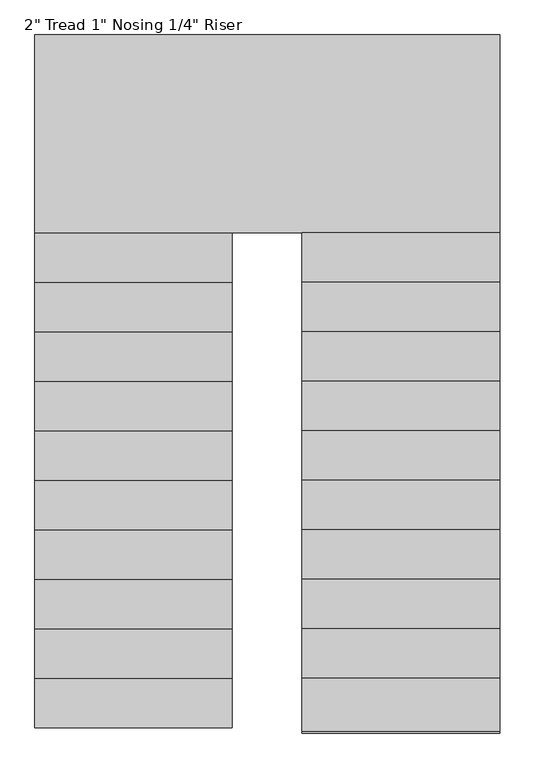
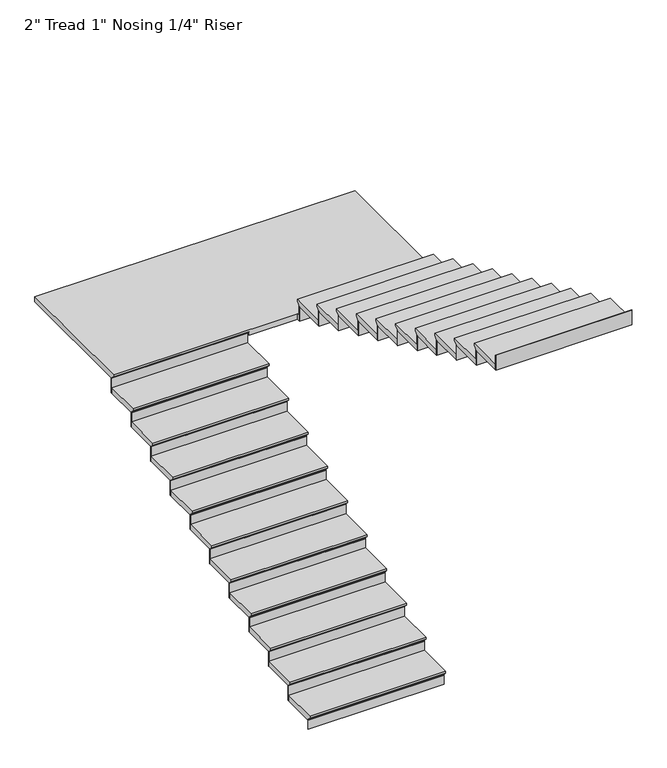
"""IFC4 building model written with IfcOpenShell, lengths in millimetres: stair flight geometry."""

from ifc_helpers import new_model, si_unit, origin, place, context, project, spatial, faceted_brep, source, transform, mapped, element, save


def stair_flight_7b3ce822(model_context):
    return source(origin(), model_context, "Body", "Brep", [
        faceted_brep([(-629.5987998, 3364.6067329, 12921.0954545), (-629.5987998, 3364.6067329, 12940.1454545), (-1845.5417538, 3364.6067329, 12940.1454545), (-1845.5417538, 3364.6067329, 12921.0954545), (-629.5987998, 3390.0067329, 12895.6954545), (-1845.5417538, 3390.0067329, 12895.6954545), (-629.5987998, 3694.8067329, 12940.1454545), (-1845.5417538, 3694.8067329, 12940.1454545), (-1845.5417538, 3390.0067329, 12889.3454545), (-1845.5417538, 3694.8067329, 12889.3454545), (-629.5987998, 3694.8067329, 12889.3454545), (-629.5987998, 3390.0067329, 12889.3454545)], [[[0, 1, 2, 3]], [[4, 0, 3, 5]], [[2, 1, 6, 7]], [[8, 9, 10, 11]], [[2, 7, 9, 8, 5, 3]], [[8, 11, 4, 5]], [[6, 1, 0, 4, 11, 10]], [[7, 6, 10, 9]]]),
        faceted_brep([(-629.5987998, 3390.0067329, 12889.3454545), (-629.5987998, 3390.0067329, 12801.6), (-629.5987998, 3396.3567329, 12801.6), (-629.5987998, 3396.3567329, 12889.3454545), (-1845.5417538, 3390.0067329, 12889.3454545), (-1845.5417538, 3396.3567329, 12889.3454545), (-1845.5417538, 3396.3567329, 12801.6), (-1845.5417538, 3390.0067329, 12801.6)], [[[0, 1, 2, 3]], [[4, 5, 6, 7]], [[1, 0, 4, 7]], [[2, 1, 7, 6]], [[3, 2, 6, 5]], [[0, 3, 5, 4]]]),
        faceted_brep([(-629.5987998, 3694.8067329, 13027.8909091), (-629.5987998, 3694.8067329, 12889.3454545), (-629.5987998, 3701.1567329, 12889.3454545), (-629.5987998, 3701.1567329, 13027.8909091), (-1845.5417538, 3694.8067329, 13027.8909091), (-1845.5417538, 3701.1567329, 13027.8909091), (-1845.5417538, 3701.1567329, 12889.3454545), (-1845.5417538, 3694.8067329, 12889.3454545)], [[[0, 1, 2, 3]], [[4, 5, 6, 7]], [[1, 0, 4, 7]], [[2, 1, 7, 6]], [[3, 2, 6, 5]], [[0, 3, 5, 4]]]),
        faceted_brep([(-1845.5417538, 3669.4067329, 13078.6909091), (-629.5987998, 3669.4067329, 13078.6909091), (-629.5987998, 3999.6067329, 13078.6909091), (-1845.5417538, 3999.6067329, 13078.6909091), (-1845.5417538, 3694.8067329, 13027.8909091), (-1845.5417538, 3999.6067329, 13027.8909091), (-629.5987998, 3999.6067329, 13027.8909091), (-629.5987998, 3694.8067329, 13027.8909091), (-1845.5417538, 3694.8067329, 13034.2409091), (-1845.5417538, 3669.4067329, 13059.6409091), (-629.5987998, 3694.8067329, 13034.2409091), (-629.5987998, 3669.4067329, 13059.6409091)], [[[0, 1, 2, 3]], [[4, 5, 6, 7]], [[0, 3, 5, 4, 8, 9]], [[4, 7, 10, 8]], [[2, 1, 11, 10, 7, 6]], [[3, 2, 6, 5]], [[11, 1, 0, 9]], [[10, 11, 9, 8]]]),
        faceted_brep([(-629.5987998, 3999.6067329, 13166.4363636), (-629.5987998, 3999.6067329, 13027.8909091), (-629.5987998, 4005.9567329, 13027.8909091), (-629.5987998, 4005.9567329, 13166.4363636), (-1845.5417538, 3999.6067329, 13166.4363636), (-1845.5417538, 4005.9567329, 13166.4363636), (-1845.5417538, 4005.9567329, 13027.8909091), (-1845.5417538, 3999.6067329, 13027.8909091)], [[[0, 1, 2, 3]], [[4, 5, 6, 7]], [[1, 0, 4, 7]], [[2, 1, 7, 6]], [[3, 2, 6, 5]], [[0, 3, 5, 4]]]),
        faceted_brep([(-1845.5417538, 3974.2067329, 13217.2363636), (-629.5987998, 3974.2067329, 13217.2363636), (-629.5987998, 4304.4067329, 13217.2363636), (-1845.5417538, 4304.4067329, 13217.2363636), (-1845.5417538, 3999.6067329, 13166.4363636), (-1845.5417538, 4304.4067329, 13166.4363636), (-629.5987998, 4304.4067329, 13166.4363636), (-629.5987998, 3999.6067329, 13166.4363636), (-1845.5417538, 3999.6067329, 13172.7863636), (-1845.5417538, 3974.2067329, 13198.1863636), (-629.5987998, 3999.6067329, 13172.7863636), (-629.5987998, 3974.2067329, 13198.1863636)], [[[0, 1, 2, 3]], [[4, 5, 6, 7]], [[0, 3, 5, 4, 8, 9]], [[4, 7, 10, 8]], [[2, 1, 11, 10, 7, 6]], [[3, 2, 6, 5]], [[11, 1, 0, 9]], [[10, 11, 9, 8]]]),
        faceted_brep([(-629.5987998, 4304.4067329, 13304.9818182), (-629.5987998, 4304.4067329, 13166.4363636), (-629.5987998, 4310.7567329, 13166.4363636), (-629.5987998, 4310.7567329, 13304.9818182), (-1845.5417538, 4304.4067329, 13304.9818182), (-1845.5417538, 4310.7567329, 13304.9818182), (-1845.5417538, 4310.7567329, 13166.4363636), (-1845.5417538, 4304.4067329, 13166.4363636)], [[[0, 1, 2, 3]], [[4, 5, 6, 7]], [[1, 0, 4, 7]], [[2, 1, 7, 6]], [[3, 2, 6, 5]], [[0, 3, 5, 4]]]),
        faceted_brep([(-1845.5417538, 4279.0067329, 13355.7818182), (-629.5987998, 4279.0067329, 13355.7818182), (-629.5987998, 4609.2067329, 13355.7818182), (-1845.5417538, 4609.2067329, 13355.7818182), (-1845.5417538, 4304.4067329, 13304.9818182), (-1845.5417538, 4609.2067329, 13304.9818182), (-629.5987998, 4609.2067329, 13304.9818182), (-629.5987998, 4304.4067329, 13304.9818182), (-1845.5417538, 4304.4067329, 13311.3318182), (-1845.5417538, 4279.0067329, 13336.7318182), (-629.5987998, 4304.4067329, 13311.3318182), (-629.5987998, 4279.0067329, 13336.7318182)], [[[0, 1, 2, 3]], [[4, 5, 6, 7]], [[0, 3, 5, 4, 8, 9]], [[4, 7, 10, 8]], [[2, 1, 11, 10, 7, 6]], [[3, 2, 6, 5]], [[11, 1, 0, 9]], [[10, 11, 9, 8]]]),
        faceted_brep([(-629.5987998, 4609.2067329, 13443.5272727), (-629.5987998, 4609.2067329, 13304.9818182), (-629.5987998, 4615.5567329, 13304.9818182), (-629.5987998, 4615.5567329, 13443.5272727), (-1845.5417538, 4609.2067329, 13443.5272727), (-1845.5417538, 4615.5567329, 13443.5272727), (-1845.5417538, 4615.5567329, 13304.9818182), (-1845.5417538, 4609.2067329, 13304.9818182)], [[[0, 1, 2, 3]], [[4, 5, 6, 7]], [[1, 0, 4, 7]], [[2, 1, 7, 6]], [[3, 2, 6, 5]], [[0, 3, 5, 4]]]),
        faceted_brep([(-1845.5417538, 4583.8067329, 13494.3272727), (-629.5987998, 4583.8067329, 13494.3272727), (-629.5987998, 4914.0067329, 13494.3272727), (-1845.5417538, 4914.0067329, 13494.3272727), (-1845.5417538, 4609.2067329, 13443.5272727), (-1845.5417538, 4914.0067329, 13443.5272727), (-629.5987998, 4914.0067329, 13443.5272727), (-629.5987998, 4609.2067329, 13443.5272727), (-1845.5417538, 4609.2067329, 13449.8772727), (-1845.5417538, 4583.8067329, 13475.2772727), (-629.5987998, 4609.2067329, 13449.8772727), (-629.5987998, 4583.8067329, 13475.2772727)], [[[0, 1, 2, 3]], [[4, 5, 6, 7]], [[0, 3, 5, 4, 8, 9]], [[4, 7, 10, 8]], [[2, 1, 11, 10, 7, 6]], [[3, 2, 6, 5]], [[11, 1, 0, 9]], [[10, 11, 9, 8]]]),
        faceted_brep([(-629.5987998, 4914.0067329, 13582.0727273), (-629.5987998, 4914.0067329, 13443.5272727), (-629.5987998, 4920.3567329, 13443.5272727), (-629.5987998, 4920.3567329, 13582.0727273), (-1845.5417538, 4914.0067329, 13582.0727273), (-1845.5417538, 4920.3567329, 13582.0727273), (-1845.5417538, 4920.3567329, 13443.5272727), (-1845.5417538, 4914.0067329, 13443.5272727)], [[[0, 1, 2, 3]], [[4, 5, 6, 7]], [[1, 0, 4, 7]], [[2, 1, 7, 6]], [[3, 2, 6, 5]], [[0, 3, 5, 4]]]),
        faceted_brep([(-1845.5417538, 4888.6067329, 13632.8727273), (-629.5987998, 4888.6067329, 13632.8727273), (-629.5987998, 5218.8067329, 13632.8727273), (-1845.5417538, 5218.8067329, 13632.8727273), (-1845.5417538, 4914.0067329, 13582.0727273), (-1845.5417538, 5218.8067329, 13582.0727273), (-629.5987998, 5218.8067329, 13582.0727273), (-629.5987998, 4914.0067329, 13582.0727273), (-1845.5417538, 4914.0067329, 13588.4227273), (-1845.5417538, 4888.6067329, 13613.8227273), (-629.5987998, 4914.0067329, 13588.4227273), (-629.5987998, 4888.6067329, 13613.8227273)], [[[0, 1, 2, 3]], [[4, 5, 6, 7]], [[0, 3, 5, 4, 8, 9]], [[4, 7, 10, 8]], [[2, 1, 11, 10, 7, 6]], [[3, 2, 6, 5]], [[11, 1, 0, 9]], [[10, 11, 9, 8]]]),
        faceted_brep([(-629.5987998, 5218.8067329, 13720.6181818), (-629.5987998, 5218.8067329, 13582.0727273), (-629.5987998, 5225.1567329, 13582.0727273), (-629.5987998, 5225.1567329, 13720.6181818), (-1845.5417538, 5218.8067329, 13720.6181818), (-1845.5417538, 5225.1567329, 13720.6181818), (-1845.5417538, 5225.1567329, 13582.0727273), (-1845.5417538, 5218.8067329, 13582.0727273)], [[[0, 1, 2, 3]], [[4, 5, 6, 7]], [[1, 0, 4, 7]], [[2, 1, 7, 6]], [[3, 2, 6, 5]], [[0, 3, 5, 4]]]),
        faceted_brep([(-1845.5417538, 5193.4067329, 13771.4181818), (-629.5987998, 5193.4067329, 13771.4181818), (-629.5987998, 5523.6067329, 13771.4181818), (-1845.5417538, 5523.6067329, 13771.4181818), (-1845.5417538, 5218.8067329, 13720.6181818), (-1845.5417538, 5523.6067329, 13720.6181818), (-629.5987998, 5523.6067329, 13720.6181818), (-629.5987998, 5218.8067329, 13720.6181818), (-1845.5417538, 5218.8067329, 13726.9681818), (-1845.5417538, 5193.4067329, 13752.3681818), (-629.5987998, 5218.8067329, 13726.9681818), (-629.5987998, 5193.4067329, 13752.3681818)], [[[0, 1, 2, 3]], [[4, 5, 6, 7]], [[0, 3, 5, 4, 8, 9]], [[4, 7, 10, 8]], [[2, 1, 11, 10, 7, 6]], [[3, 2, 6, 5]], [[11, 1, 0, 9]], [[10, 11, 9, 8]]]),
        faceted_brep([(-629.5987998, 5523.6067329, 13859.1636364), (-629.5987998, 5523.6067329, 13720.6181818), (-629.5987998, 5529.9567329, 13720.6181818), (-629.5987998, 5529.9567329, 13859.1636364), (-1845.5417538, 5523.6067329, 13859.1636364), (-1845.5417538, 5529.9567329, 13859.1636364), (-1845.5417538, 5529.9567329, 13720.6181818), (-1845.5417538, 5523.6067329, 13720.6181818)], [[[0, 1, 2, 3]], [[4, 5, 6, 7]], [[1, 0, 4, 7]], [[2, 1, 7, 6]], [[3, 2, 6, 5]], [[0, 3, 5, 4]]]),
        faceted_brep([(-1845.5417538, 5498.2067329, 13909.9636364), (-629.5987998, 5498.2067329, 13909.9636364), (-629.5987998, 5828.4067329, 13909.9636364), (-1845.5417538, 5828.4067329, 13909.9636364), (-1845.5417538, 5523.6067329, 13859.1636364), (-1845.5417538, 5828.4067329, 13859.1636364), (-629.5987998, 5828.4067329, 13859.1636364), (-629.5987998, 5523.6067329, 13859.1636364), (-1845.5417538, 5523.6067329, 13865.5136364), (-1845.5417538, 5498.2067329, 13890.9136364), (-629.5987998, 5523.6067329, 13865.5136364), (-629.5987998, 5498.2067329, 13890.9136364)], [[[0, 1, 2, 3]], [[4, 5, 6, 7]], [[0, 3, 5, 4, 8, 9]], [[4, 7, 10, 8]], [[2, 1, 11, 10, 7, 6]], [[3, 2, 6, 5]], [[11, 1, 0, 9]], [[10, 11, 9, 8]]]),
        faceted_brep([(-629.5987998, 5828.4067329, 13997.7090909), (-629.5987998, 5828.4067329, 13859.1636364), (-629.5987998, 5834.7567329, 13859.1636364), (-629.5987998, 5834.7567329, 13997.7090909), (-1845.5417538, 5828.4067329, 13997.7090909), (-1845.5417538, 5834.7567329, 13997.7090909), (-1845.5417538, 5834.7567329, 13859.1636364), (-1845.5417538, 5828.4067329, 13859.1636364)], [[[0, 1, 2, 3]], [[4, 5, 6, 7]], [[1, 0, 4, 7]], [[2, 1, 7, 6]], [[3, 2, 6, 5]], [[0, 3, 5, 4]]]),
        faceted_brep([(-1845.5417538, 5803.0067329, 14048.5090909), (-629.5987998, 5803.0067329, 14048.5090909), (-629.5987998, 6133.2067329, 14048.5090909), (-1845.5417538, 6133.2067329, 14048.5090909), (-1845.5417538, 5828.4067329, 13997.7090909), (-1845.5417538, 6133.2067329, 13997.7090909), (-629.5987998, 6133.2067329, 13997.7090909), (-629.5987998, 5828.4067329, 13997.7090909), (-1845.5417538, 5828.4067329, 14004.0590909), (-1845.5417538, 5803.0067329, 14029.4590909), (-629.5987998, 5828.4067329, 14004.0590909), (-629.5987998, 5803.0067329, 14029.4590909)], [[[0, 1, 2, 3]], [[4, 5, 6, 7]], [[0, 3, 5, 4, 8, 9]], [[4, 7, 10, 8]], [[2, 1, 11, 10, 7, 6]], [[3, 2, 6, 5]], [[11, 1, 0, 9]], [[10, 11, 9, 8]]]),
        faceted_brep([(-629.5987998, 6133.2067329, 14136.2545455), (-629.5987998, 6133.2067329, 13997.7090909), (-629.5987998, 6139.5567329, 13997.7090909), (-629.5987998, 6139.5567329, 14136.2545455), (-1845.5417538, 6133.2067329, 14136.2545455), (-1845.5417538, 6139.5567329, 14136.2545455), (-1845.5417538, 6139.5567329, 13997.7090909), (-1845.5417538, 6133.2067329, 13997.7090909)], [[[0, 1, 2, 3]], [[4, 5, 6, 7]], [[1, 0, 4, 7]], [[2, 1, 7, 6]], [[3, 2, 6, 5]], [[0, 3, 5, 4]]]),
        faceted_brep([(-1845.5417538, 6107.8067329, 14187.0545455), (-629.5987998, 6107.8067329, 14187.0545455), (-629.5987998, 6438.0067329, 14187.0545455), (-1845.5417538, 6438.0067329, 14187.0545455), (-1845.5417538, 6133.2067329, 14136.2545455), (-1845.5417538, 6438.0067329, 14136.2545455), (-629.5987998, 6438.0067329, 14136.2545455), (-629.5987998, 6133.2067329, 14136.2545455), (-1845.5417538, 6133.2067329, 14142.6045455), (-1845.5417538, 6107.8067329, 14168.0045455), (-629.5987998, 6133.2067329, 14142.6045455), (-629.5987998, 6107.8067329, 14168.0045455)], [[[0, 1, 2, 3]], [[4, 5, 6, 7]], [[0, 3, 5, 4, 8, 9]], [[4, 7, 10, 8]], [[2, 1, 11, 10, 7, 6]], [[3, 2, 6, 5]], [[11, 1, 0, 9]], [[10, 11, 9, 8]]]),
        faceted_brep([(-629.5987998, 6438.0067329, 14274.8), (-629.5987998, 6438.0067329, 14136.2545455), (-629.5987998, 6444.3567329, 14136.2545455), (-629.5987998, 6444.3567329, 14274.8), (-1845.5417538, 6438.0067329, 14274.8), (-1845.5417538, 6444.3567329, 14274.8), (-1845.5417538, 6444.3567329, 14136.2545455), (-1845.5417538, 6438.0067329, 14136.2545455)], [[[0, 1, 2, 3]], [[4, 5, 6, 7]], [[1, 0, 4, 7]], [[2, 1, 7, 6]], [[3, 2, 6, 5]], [[0, 3, 5, 4]]]),
        faceted_brep([(1021.4012085, 6387.2067329, 14325.6), (1021.4012085, 7631.8067329, 14325.6), (-1845.5417538, 7631.8067329, 14325.6), (-1845.5417538, 6412.6067329, 14325.6), (-197.7987915, 6412.6067329, 14325.6), (-197.7987915, 6387.2067329, 14325.6), (1021.4012085, 7631.8067329, 14274.8), (1021.4012085, 6387.2067329, 14274.8), (-197.7987915, 6387.2067329, 14274.8), (-197.7987915, 6412.6067329, 14274.8), (-629.5987998, 6412.6067329, 14274.8), (-629.5987998, 6438.0067329, 14274.8), (-1845.5417538, 6438.0067329, 14274.8), (-1845.5417538, 7631.8067329, 14274.8), (-629.5987998, 6438.0067329, 14281.15), (-1845.5417538, 6438.0067329, 14281.15), (-1845.5417538, 6412.6067329, 14306.55), (-629.5987998, 6412.6067329, 14306.55)], [[[0, 1, 2, 3, 4, 5]], [[6, 7, 8, 9, 10, 11, 12, 13]], [[1, 0, 7, 6]], [[2, 1, 6, 13]], [[12, 11, 14, 15]], [[4, 3, 16, 17, 10, 9]], [[5, 4, 9, 8]], [[0, 5, 8, 7]], [[16, 15, 14, 17]], [[3, 2, 13, 12, 15, 16]], [[11, 10, 17, 14]]]),
        faceted_brep([(-197.7987915, 6387.2067329, 14413.3454545), (-197.7987915, 6387.2067329, 14274.8), (-197.7987915, 6380.8567329, 14274.8), (-197.7987915, 6380.8567329, 14413.3454545), (1021.4012085, 6387.2067329, 14413.3454545), (1021.4012085, 6380.8567329, 14413.3454545), (1021.4012085, 6380.8567329, 14274.8), (1021.4012085, 6387.2067329, 14274.8)], [[[0, 1, 2, 3]], [[4, 5, 6, 7]], [[1, 0, 4, 7]], [[2, 1, 7, 6]], [[3, 2, 6, 5]], [[0, 3, 5, 4]]]),
        faceted_brep([(1021.4012085, 6412.6067329, 14464.1454545), (-197.7987915, 6412.6067329, 14464.1454545), (-197.7987915, 6082.4067329, 14464.1454545), (1021.4012085, 6082.4067329, 14464.1454545), (1021.4012085, 6387.2067329, 14413.3454545), (1021.4012085, 6082.4067329, 14413.3454545), (-197.7987915, 6082.4067329, 14413.3454545), (-197.7987915, 6387.2067329, 14413.3454545), (1021.4012085, 6387.2067329, 14419.6954545), (1021.4012085, 6412.6067329, 14445.0954545), (-197.7987915, 6387.2067329, 14419.6954545), (-197.7987915, 6412.6067329, 14445.0954545)], [[[0, 1, 2, 3]], [[4, 5, 6, 7]], [[0, 3, 5, 4, 8, 9]], [[4, 7, 10, 8]], [[2, 1, 11, 10, 7, 6]], [[3, 2, 6, 5]], [[11, 1, 0, 9]], [[10, 11, 9, 8]]]),
        faceted_brep([(-197.7987915, 6082.4067329, 14551.8909091), (-197.7987915, 6082.4067329, 14413.3454545), (-197.7987915, 6076.0567329, 14413.3454545), (-197.7987915, 6076.0567329, 14551.8909091), (1021.4012085, 6082.4067329, 14551.8909091), (1021.4012085, 6076.0567329, 14551.8909091), (1021.4012085, 6076.0567329, 14413.3454545), (1021.4012085, 6082.4067329, 14413.3454545)], [[[0, 1, 2, 3]], [[4, 5, 6, 7]], [[1, 0, 4, 7]], [[2, 1, 7, 6]], [[3, 2, 6, 5]], [[0, 3, 5, 4]]]),
        faceted_brep([(1021.4012085, 6107.8067329, 14602.6909091), (-197.7987915, 6107.8067329, 14602.6909091), (-197.7987915, 5777.6067329, 14602.6909091), (1021.4012085, 5777.6067329, 14602.6909091), (1021.4012085, 6082.4067329, 14551.8909091), (1021.4012085, 5777.6067329, 14551.8909091), (-197.7987915, 5777.6067329, 14551.8909091), (-197.7987915, 6082.4067329, 14551.8909091), (1021.4012085, 6082.4067329, 14558.2409091), (1021.4012085, 6107.8067329, 14583.6409091), (-197.7987915, 6082.4067329, 14558.2409091), (-197.7987915, 6107.8067329, 14583.6409091)], [[[0, 1, 2, 3]], [[4, 5, 6, 7]], [[0, 3, 5, 4, 8, 9]], [[4, 7, 10, 8]], [[2, 1, 11, 10, 7, 6]], [[3, 2, 6, 5]], [[11, 1, 0, 9]], [[10, 11, 9, 8]]]),
        faceted_brep([(-197.7987915, 5777.6067329, 14690.4363636), (-197.7987915, 5777.6067329, 14551.8909091), (-197.7987915, 5771.2567329, 14551.8909091), (-197.7987915, 5771.2567329, 14690.4363636), (1021.4012085, 5777.6067329, 14690.4363636), (1021.4012085, 5771.2567329, 14690.4363636), (1021.4012085, 5771.2567329, 14551.8909091), (1021.4012085, 5777.6067329, 14551.8909091)], [[[0, 1, 2, 3]], [[4, 5, 6, 7]], [[1, 0, 4, 7]], [[2, 1, 7, 6]], [[3, 2, 6, 5]], [[0, 3, 5, 4]]]),
        faceted_brep([(1021.4012085, 5803.0067329, 14741.2363636), (-197.7987915, 5803.0067329, 14741.2363636), (-197.7987915, 5472.8067329, 14741.2363636), (1021.4012085, 5472.8067329, 14741.2363636), (1021.4012085, 5777.6067329, 14690.4363636), (1021.4012085, 5472.8067329, 14690.4363636), (-197.7987915, 5472.8067329, 14690.4363636), (-197.7987915, 5777.6067329, 14690.4363636), (1021.4012085, 5777.6067329, 14696.7863636), (1021.4012085, 5803.0067329, 14722.1863636), (-197.7987915, 5777.6067329, 14696.7863636), (-197.7987915, 5803.0067329, 14722.1863636)], [[[0, 1, 2, 3]], [[4, 5, 6, 7]], [[0, 3, 5, 4, 8, 9]], [[4, 7, 10, 8]], [[2, 1, 11, 10, 7, 6]], [[3, 2, 6, 5]], [[11, 1, 0, 9]], [[10, 11, 9, 8]]]),
        faceted_brep([(-197.7987915, 5472.8067329, 14828.9818182), (-197.7987915, 5472.8067329, 14690.4363636), (-197.7987915, 5466.4567329, 14690.4363636), (-197.7987915, 5466.4567329, 14828.9818182), (1021.4012085, 5472.8067329, 14828.9818182), (1021.4012085, 5466.4567329, 14828.9818182), (1021.4012085, 5466.4567329, 14690.4363636), (1021.4012085, 5472.8067329, 14690.4363636)], [[[0, 1, 2, 3]], [[4, 5, 6, 7]], [[1, 0, 4, 7]], [[2, 1, 7, 6]], [[3, 2, 6, 5]], [[0, 3, 5, 4]]]),
        faceted_brep([(1021.4012085, 5498.2067329, 14879.7818182), (-197.7987915, 5498.2067329, 14879.7818182), (-197.7987915, 5168.0067329, 14879.7818182), (1021.4012085, 5168.0067329, 14879.7818182), (1021.4012085, 5472.8067329, 14828.9818182), (1021.4012085, 5168.0067329, 14828.9818182), (-197.7987915, 5168.0067329, 14828.9818182), (-197.7987915, 5472.8067329, 14828.9818182), (1021.4012085, 5472.8067329, 14835.3318182), (1021.4012085, 5498.2067329, 14860.7318182), (-197.7987915, 5472.8067329, 14835.3318182), (-197.7987915, 5498.2067329, 14860.7318182)], [[[0, 1, 2, 3]], [[4, 5, 6, 7]], [[0, 3, 5, 4, 8, 9]], [[4, 7, 10, 8]], [[2, 1, 11, 10, 7, 6]], [[3, 2, 6, 5]], [[11, 1, 0, 9]], [[10, 11, 9, 8]]]),
        faceted_brep([(-197.7987915, 5168.0067329, 14967.5272727), (-197.7987915, 5168.0067329, 14828.9818182), (-197.7987915, 5161.6567329, 14828.9818182), (-197.7987915, 5161.6567329, 14967.5272727), (1021.4012085, 5168.0067329, 14967.5272727), (1021.4012085, 5161.6567329, 14967.5272727), (1021.4012085, 5161.6567329, 14828.9818182), (1021.4012085, 5168.0067329, 14828.9818182)], [[[0, 1, 2, 3]], [[4, 5, 6, 7]], [[1, 0, 4, 7]], [[2, 1, 7, 6]], [[3, 2, 6, 5]], [[0, 3, 5, 4]]]),
        faceted_brep([(1021.4012085, 5193.4067329, 15018.3272727), (-197.7987915, 5193.4067329, 15018.3272727), (-197.7987915, 4863.2067329, 15018.3272727), (1021.4012085, 4863.2067329, 15018.3272727), (1021.4012085, 5168.0067329, 14967.5272727), (1021.4012085, 4863.2067329, 14967.5272727), (-197.7987915, 4863.2067329, 14967.5272727), (-197.7987915, 5168.0067329, 14967.5272727), (1021.4012085, 5168.0067329, 14973.8772727), (1021.4012085, 5193.4067329, 14999.2772727), (-197.7987915, 5168.0067329, 14973.8772727), (-197.7987915, 5193.4067329, 14999.2772727)], [[[0, 1, 2, 3]], [[4, 5, 6, 7]], [[0, 3, 5, 4, 8, 9]], [[4, 7, 10, 8]], [[2, 1, 11, 10, 7, 6]], [[3, 2, 6, 5]], [[11, 1, 0, 9]], [[10, 11, 9, 8]]]),
        faceted_brep([(-197.7987915, 4863.2067329, 15106.0727273), (-197.7987915, 4863.2067329, 14967.5272727), (-197.7987915, 4856.8567329, 14967.5272727), (-197.7987915, 4856.8567329, 15106.0727273), (1021.4012085, 4863.2067329, 15106.0727273), (1021.4012085, 4856.8567329, 15106.0727273), (1021.4012085, 4856.8567329, 14967.5272727), (1021.4012085, 4863.2067329, 14967.5272727)], [[[0, 1, 2, 3]], [[4, 5, 6, 7]], [[1, 0, 4, 7]], [[2, 1, 7, 6]], [[3, 2, 6, 5]], [[0, 3, 5, 4]]]),
        faceted_brep([(1021.4012085, 4888.6067329, 15156.8727273), (-197.7987915, 4888.6067329, 15156.8727273), (-197.7987915, 4558.4067329, 15156.8727273), (1021.4012085, 4558.4067329, 15156.8727273), (1021.4012085, 4863.2067329, 15106.0727273), (1021.4012085, 4558.4067329, 15106.0727273), (-197.7987915, 4558.4067329, 15106.0727273), (-197.7987915, 4863.2067329, 15106.0727273), (1021.4012085, 4863.2067329, 15112.4227273), (1021.4012085, 4888.6067329, 15137.8227273), (-197.7987915, 4863.2067329, 15112.4227273), (-197.7987915, 4888.6067329, 15137.8227273)], [[[0, 1, 2, 3]], [[4, 5, 6, 7]], [[0, 3, 5, 4, 8, 9]], [[4, 7, 10, 8]], [[2, 1, 11, 10, 7, 6]], [[3, 2, 6, 5]], [[11, 1, 0, 9]], [[10, 11, 9, 8]]]),
        faceted_brep([(-197.7987915, 4558.4067329, 15244.6181818), (-197.7987915, 4558.4067329, 15106.0727273), (-197.7987915, 4552.0567329, 15106.0727273), (-197.7987915, 4552.0567329, 15244.6181818), (1021.4012085, 4558.4067329, 15244.6181818), (1021.4012085, 4552.0567329, 15244.6181818), (1021.4012085, 4552.0567329, 15106.0727273), (1021.4012085, 4558.4067329, 15106.0727273)], [[[0, 1, 2, 3]], [[4, 5, 6, 7]], [[1, 0, 4, 7]], [[2, 1, 7, 6]], [[3, 2, 6, 5]], [[0, 3, 5, 4]]]),
        faceted_brep([(1021.4012085, 4583.8067329, 15295.4181818), (-197.7987915, 4583.8067329, 15295.4181818), (-197.7987915, 4253.6067329, 15295.4181818), (1021.4012085, 4253.6067329, 15295.4181818), (1021.4012085, 4558.4067329, 15244.6181818), (1021.4012085, 4253.6067329, 15244.6181818), (-197.7987915, 4253.6067329, 15244.6181818), (-197.7987915, 4558.4067329, 15244.6181818), (1021.4012085, 4558.4067329, 15250.9681818), (1021.4012085, 4583.8067329, 15276.3681818), (-197.7987915, 4558.4067329, 15250.9681818), (-197.7987915, 4583.8067329, 15276.3681818)], [[[0, 1, 2, 3]], [[4, 5, 6, 7]], [[0, 3, 5, 4, 8, 9]], [[4, 7, 10, 8]], [[2, 1, 11, 10, 7, 6]], [[3, 2, 6, 5]], [[11, 1, 0, 9]], [[10, 11, 9, 8]]]),
        faceted_brep([(-197.7987915, 4253.6067329, 15383.1636364), (-197.7987915, 4253.6067329, 15244.6181818), (-197.7987915, 4247.2567329, 15244.6181818), (-197.7987915, 4247.2567329, 15383.1636364), (1021.4012085, 4253.6067329, 15383.1636364), (1021.4012085, 4247.2567329, 15383.1636364), (1021.4012085, 4247.2567329, 15244.6181818), (1021.4012085, 4253.6067329, 15244.6181818)], [[[0, 1, 2, 3]], [[4, 5, 6, 7]], [[1, 0, 4, 7]], [[2, 1, 7, 6]], [[3, 2, 6, 5]], [[0, 3, 5, 4]]]),
        faceted_brep([(1021.4012085, 4279.0067329, 15433.9636364), (-197.7987915, 4279.0067329, 15433.9636364), (-197.7987915, 3948.8067329, 15433.9636364), (1021.4012085, 3948.8067329, 15433.9636364), (1021.4012085, 4253.6067329, 15383.1636364), (1021.4012085, 3948.8067329, 15383.1636364), (-197.7987915, 3948.8067329, 15383.1636364), (-197.7987915, 4253.6067329, 15383.1636364), (1021.4012085, 4253.6067329, 15389.5136364), (1021.4012085, 4279.0067329, 15414.9136364), (-197.7987915, 4253.6067329, 15389.5136364), (-197.7987915, 4279.0067329, 15414.9136364)], [[[0, 1, 2, 3]], [[4, 5, 6, 7]], [[0, 3, 5, 4, 8, 9]], [[4, 7, 10, 8]], [[2, 1, 11, 10, 7, 6]], [[3, 2, 6, 5]], [[11, 1, 0, 9]], [[10, 11, 9, 8]]]),
        faceted_brep([(-197.7987915, 3948.8067329, 15521.7090909), (-197.7987915, 3948.8067329, 15383.1636364), (-197.7987915, 3942.4567329, 15383.1636364), (-197.7987915, 3942.4567329, 15521.7090909), (1021.4012085, 3948.8067329, 15521.7090909), (1021.4012085, 3942.4567329, 15521.7090909), (1021.4012085, 3942.4567329, 15383.1636364), (1021.4012085, 3948.8067329, 15383.1636364)], [[[0, 1, 2, 3]], [[4, 5, 6, 7]], [[1, 0, 4, 7]], [[2, 1, 7, 6]], [[3, 2, 6, 5]], [[0, 3, 5, 4]]]),
        faceted_brep([(1021.4012085, 3974.2067329, 15572.5090909), (-197.7987915, 3974.2067329, 15572.5090909), (-197.7987915, 3644.0067329, 15572.5090909), (1021.4012085, 3644.0067329, 15572.5090909), (1021.4012085, 3948.8067329, 15521.7090909), (1021.4012085, 3644.0067329, 15521.7090909), (-197.7987915, 3644.0067329, 15521.7090909), (-197.7987915, 3948.8067329, 15521.7090909), (1021.4012085, 3948.8067329, 15528.0590909), (1021.4012085, 3974.2067329, 15553.4590909), (-197.7987915, 3948.8067329, 15528.0590909), (-197.7987915, 3974.2067329, 15553.4590909)], [[[0, 1, 2, 3]], [[4, 5, 6, 7]], [[0, 3, 5, 4, 8, 9]], [[4, 7, 10, 8]], [[2, 1, 11, 10, 7, 6]], [[3, 2, 6, 5]], [[11, 1, 0, 9]], [[10, 11, 9, 8]]]),
        faceted_brep([(-197.7987915, 3644.0067329, 15660.2545455), (-197.7987915, 3644.0067329, 15521.7090909), (-197.7987915, 3637.6567329, 15521.7090909), (-197.7987915, 3637.6567329, 15660.2545455), (1021.4012085, 3644.0067329, 15660.2545455), (1021.4012085, 3637.6567329, 15660.2545455), (1021.4012085, 3637.6567329, 15521.7090909), (1021.4012085, 3644.0067329, 15521.7090909)], [[[0, 1, 2, 3]], [[4, 5, 6, 7]], [[1, 0, 4, 7]], [[2, 1, 7, 6]], [[3, 2, 6, 5]], [[0, 3, 5, 4]]]),
        faceted_brep([(-197.7987915, 3339.2067329, 15798.8), (-197.7987915, 3339.2067329, 15660.2545455), (-197.7987915, 3332.8567329, 15660.2545455), (-197.7987915, 3332.8567329, 15798.8), (1021.4012085, 3339.2067329, 15798.8), (1021.4012085, 3332.8567329, 15798.8), (1021.4012085, 3332.8567329, 15660.2545455), (1021.4012085, 3339.2067329, 15660.2545455)], [[[0, 1, 2, 3]], [[4, 5, 6, 7]], [[1, 0, 4, 7]], [[2, 1, 7, 6]], [[3, 2, 6, 5]], [[0, 3, 5, 4]]]),
        faceted_brep([(1021.4012085, 3669.4067329, 15711.0545455), (-197.7987915, 3669.4067329, 15711.0545455), (-197.7987915, 3339.2067329, 15711.0545455), (1021.4012085, 3339.2067329, 15711.0545455), (1021.4012085, 3644.0067329, 15660.2545455), (1021.4012085, 3339.2067329, 15660.2545455), (-197.7987915, 3339.2067329, 15660.2545455), (-197.7987915, 3644.0067329, 15660.2545455), (1021.4012085, 3644.0067329, 15666.6045455), (1021.4012085, 3669.4067329, 15692.0045455), (-197.7987915, 3644.0067329, 15666.6045455), (-197.7987915, 3669.4067329, 15692.0045455)], [[[0, 1, 2, 3]], [[4, 5, 6, 7]], [[0, 3, 5, 4, 8, 9]], [[4, 7, 10, 8]], [[2, 1, 11, 10, 7, 6]], [[3, 2, 6, 5]], [[11, 1, 0, 9]], [[10, 11, 9, 8]]]),
    ])


if __name__ == "__main__":
    model = new_model("IFC4")
    model_context = context("Model", 3, world=origin())
    ifc_project = project(units=[si_unit("LENGTHUNIT", "METRE", prefix="MILLI")], contexts=[model_context])
    site = spatial("IfcSite", under=ifc_project)
    building = spatial("IfcBuilding", under=site)
    placement = place(None, origin())
    stair_flight_shape = stair_flight_7b3ce822(model_context)
    element("IfcStairFlight", 1, ObjectType="2\" Tread 1\" Nosing 1/4\" Riser", at=placement, inside=building, context=model_context, shape_type="MappedRepresentation", body=[
        mapped(stair_flight_shape, transform((0.0, 0.0, 0.0), x_axis=(1.0, 0.0, 0.0), y_axis=(0.0, 1.0, 0.0), z_axis=(0.0, 0.0, 1.0))),
    ])
    save(model, "model.ifc")
